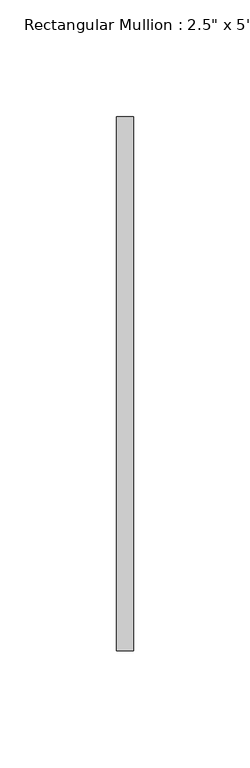
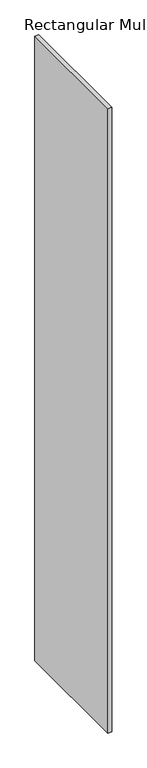
"""IFC4 building model written with IfcOpenShell, lengths in millimetres: member geometry."""

from ifc_helpers import new_model, si_unit, frame, origin, place, context, project, spatial, polyline, outline, extrude, source, transform, mapped, element, save


def member_897fe9bb(model_context):
    return source(origin(), model_context, "Body", "SweptSolid", [
        extrude(outline(polyline([(3.6195, 114.3), (3.6195, -114.3), (-3.6195, -114.3), (-3.6195, 114.3), (3.6195, 114.3)])), frame((0.0, 0.0, -1193.8), z_axis=(0.0, 0.0, 1.0), x_axis=(1.0, 0.0, 0.0)), (0.0, 0.0, 1.0), 1193.8),
    ])


if __name__ == "__main__":
    model = new_model("IFC4")
    model_context = context("Model", 3, world=origin())
    ifc_project = project(units=[si_unit("LENGTHUNIT", "METRE", prefix="MILLI")], contexts=[model_context])
    site = spatial("IfcSite", under=ifc_project)
    building = spatial("IfcBuilding", under=site)
    placement = place(None, origin())
    member_shape = member_897fe9bb(model_context)
    element("IfcMember", 1, ObjectType="Rectangular Mullion : 2.5\" x 5\" rectangular", at=placement, inside=building, context=model_context, shape_type="MappedRepresentation", body=[
        mapped(member_shape, transform((0.0, 0.0, 0.0), x_axis=(1.0, 0.0, 0.0), y_axis=(0.0, 1.0, 0.0), z_axis=(0.0, 0.0, 1.0))),
    ])
    save(model, "model.ifc")

# Revit data of these elements
# Type "Rectangular Mullion : 2.5\" x 5\" rectangular"
#   built-in parameter 1007304 = 0.75 (stored number, unit not read)
#   built-in parameter 1007301 = 0.011875 (stored number, unit not read)
#   built-in parameter 1007300 = 0.011875 (stored number, unit not read)
# Element 1 (IfcMember, "Rectangular Mullion : 2.5\" x 5\" rectangular")
#   Materials on its faces: "WINDOW GLASS MATERIAL"
# Materials
#   "WINDOW GLASS MATERIAL": class "Generic", colour RGB 120 120 120, transparency 0, Cost = 0
